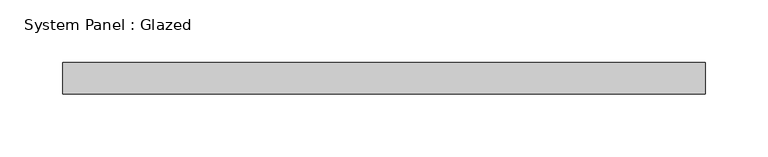
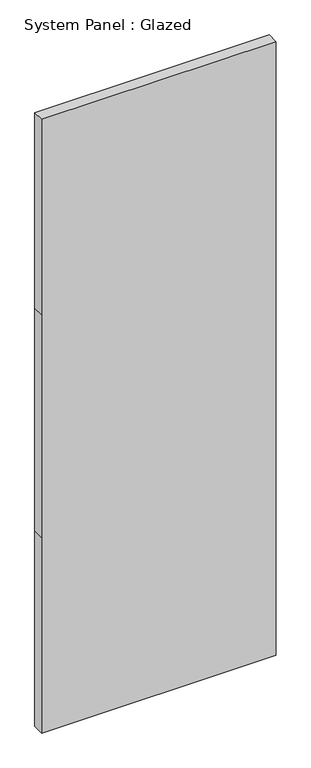
"""IFC4 building model written with IfcOpenShell, lengths in millimetres: plate geometry, System Panel : Glazed."""

from ifc_helpers import new_model, si_unit, frame, origin, place, context, project, spatial, polyline, outline, extrude, source, transform, mapped, element, save


def system_panel_glazed_f555cb13(model_context):
    return source(origin(), model_context, "Body", "SweptSolid", [
        extrude(outline(polyline([(0.0, -257.175), (0.0, 257.175), (452.9666667, 257.175), (969.4333333, 257.175), (1422.4, 257.175), (1422.4, -257.175), (969.4333333, -257.175), (452.9666667, -257.175), (0.0, -257.175)])), frame((0.0, 19.05, 0.0), z_axis=(0.0, 1.0, 0.0), x_axis=(0.0, 0.0, 1.0)), (0.0, 0.0, 1.0), 25.4),
    ])


if __name__ == "__main__":
    model = new_model("IFC4")
    model_context = context("Model", 3, world=origin())
    ifc_project = project(units=[si_unit("LENGTHUNIT", "METRE", prefix="MILLI")], contexts=[model_context])
    site = spatial("IfcSite", under=ifc_project)
    building = spatial("IfcBuilding", under=site)
    placement = place(None, origin())
    system_panel_glazed_shape = system_panel_glazed_f555cb13(model_context)
    element("IfcPlate", 1, ObjectType="System Panel : Glazed", at=placement, inside=building, context=model_context, shape_type="MappedRepresentation", body=[
        mapped(system_panel_glazed_shape, transform((0.0, 0.0, 0.0), x_axis=(1.0, 0.0, 0.0), y_axis=(0.0, 1.0, 0.0), z_axis=(0.0, 0.0, 1.0))),
    ])
    save(model, "model.ifc")

# Revit data of these elements
# Type "System Panel : Glazed"
#   Construction Type Id = "GSP4R"
#   Analytic Construction = "1/8 in Pilkington single glazing"
#   Visual Light Transmittance = 0.9
#   Solar Heat Gain Coefficient = 0.86
#   Heat Transfer Coefficient (U) = 1.18115 BTU/(h·ft²·°F)
#   Define Thermal Properties by = 1
# Element 1 (IfcPlate, "System Panel : Glazed")
#   Materials on its faces: "Glass"
# Materials
#   "Glass": class "Glass", colour RGB 0 128 192, transparency 0.75, Description = "Soda Lime Glass", Cost = 0
